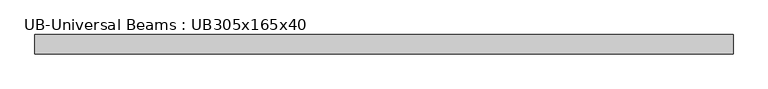
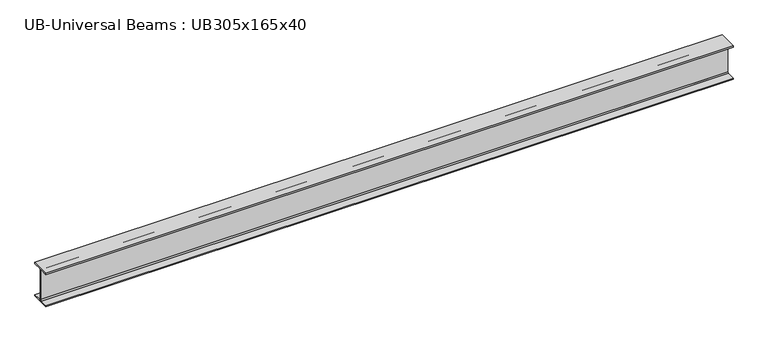
"""IFC4 building model written with IfcOpenShell, lengths in millimetres: beam geometry, UB-Universal Beams : UB305x165x40."""

from ifc_helpers import new_model, si_unit, point, frame, frame_2d, origin, place, context, project, spatial, polyline, circle_curve, trimmed, segment, composite_curve, outline, extrude, source, transform, mapped, element, save


def ub_universal_beams_ub305x165x40_15f88fa9(model_context):
    return source(origin(), model_context, "Body", "SweptSolid", [
        extrude(outline(composite_curve([segment(polyline([(82.5, -141.5), (82.5, -151.7), (-82.5, -151.7), (-82.5, -141.5), (-11.9, -141.5)]), True, "CONTINUOUS"), segment(trimmed(circle_curve(frame_2d((-11.9, -132.6)), 8.9), [point((-11.9, -141.5))], [point((-3.0, -132.6))], True, "CARTESIAN"), True, "CONTINUOUS"), segment(polyline([(-3.0, -132.6), (-3.0, 132.6)]), True, "CONTINUOUS"), segment(trimmed(circle_curve(frame_2d((-11.9, 132.6)), 8.9), [point((-3.0, 132.6))], [point((-11.9, 141.5))], True, "CARTESIAN"), True, "CONTINUOUS"), segment(polyline([(-11.9, 141.5), (-82.5, 141.5), (-82.5, 151.7), (82.5, 151.7), (82.5, 141.5), (11.9, 141.5)]), True, "CONTINUOUS"), segment(trimmed(circle_curve(frame_2d((11.9, 132.6)), 8.9), [point((11.9, 141.5))], [point((3.0, 132.6))], True, "CARTESIAN"), True, "CONTINUOUS"), segment(polyline([(3.0, 132.6), (3.0, -132.6)]), True, "CONTINUOUS"), segment(trimmed(circle_curve(frame_2d((11.9, -132.6)), 8.9), [point((3.0, -132.6))], [point((11.9, -141.5))], True, "CARTESIAN"), True, "CONTINUOUS"), segment(polyline([(11.9, -141.5), (82.5, -141.5)]), True, "CONTINUOUS")], self_intersect=False)), frame((-2952.8, 0.0, 0.0), z_axis=(1.0, 0.0, 0.0), x_axis=(0.0, 1.0, 0.0)), (0.0, 0.0, 1.0), 5905.6),
    ])


if __name__ == "__main__":
    model = new_model("IFC4")
    model_context = context("Model", 3, world=origin())
    ifc_project = project(units=[si_unit("LENGTHUNIT", "METRE", prefix="MILLI")], contexts=[model_context])
    site = spatial("IfcSite", under=ifc_project)
    building = spatial("IfcBuilding", under=site)
    placement = place(None, origin())
    ub_universal_beams_ub305x165x40_shape = ub_universal_beams_ub305x165x40_15f88fa9(model_context)
    element("IfcBeam", 1, ObjectType="UB-Universal Beams : UB305x165x40", at=placement, inside=building, context=model_context, shape_type="MappedRepresentation", body=[
        mapped(ub_universal_beams_ub305x165x40_shape, transform((0.0, 0.0, 0.0), x_axis=(1.0, 0.0, 0.0), y_axis=(0.0, 1.0, 0.0), z_axis=(0.0, 0.0, 1.0))),
    ])
    save(model, "model.ifc")

# Revit data of these elements
# Type "UB-Universal Beams : UB305x165x40"
#   Section Name Key = "UB305X165X40"
#   Width = 16.5 cm
#   Web Thickness = 0.6 cm
#   Web Fillet = 0.89 cm
#   Warping Constant = 164000.0 cm⁶
#   Torsional Moment of Inertia = 14.70 cm⁴
#   Section Area = 51.3 cm²
#   Plastic Modulus weak axis = 142.0 cm³
#   Plastic Modulus strong axis = 623.0 cm³
#   Nominal Weight = 40.2999 kgf/m
#   Moment of Inertia weak axis = 764.00 cm⁴
#   Moment of Inertia strong axis = 8503.00 cm⁴
#   Height = 30.34 cm
#   Flange Thickness = 1.02 cm
#   Elastic Modulus weak axis = 92.6 cm³
#   Elastic Modulus strong axis = 560.0 cm³
#   Centroid Vertical = 15.17 cm
#   Centroid Horizontal = 8.25 cm
#   Bolt Spacing = 9.0 cm
#   Length [instance default] = 1500 mm
#   Structural Material [instance default] = Metal - Steel 43-275
#   Type Comments = ""
#   Assembly Code = ""
# Element 1 (IfcBeam, "UB-Universal Beams : UB305x165x40")
#   Materials on its faces: "Metal - Steel 43-275"
# Materials
#   "Metal - Steel 43-275": class "Metal", colour RGB 247 247 247, transparency 0, Cost = 0
